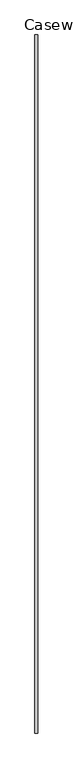
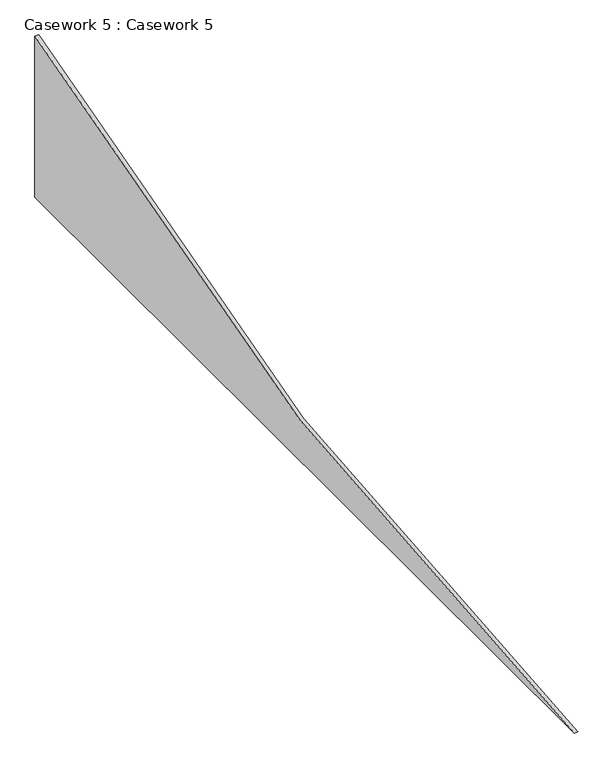
"""IFC4 building model written with IfcOpenShell, lengths in millimetres: furniture geometry, Casework 5 : Casework 5."""

from ifc_helpers import new_model, si_unit, point, frame, frame_2d, origin, place, context, project, spatial, polyline, circle_curve, trimmed, segment, composite_curve, outline, extrude, source, transform, mapped, element, save


def casework_5_casework_5_bcf4e650(model_context):
    return source(origin(), model_context, "Body", "SweptSolid", [
        extrude(outline(composite_curve([segment(polyline([(12368.6757925, 4114.8), (-432.9242075, 4114.8)]), True, "CONTINUOUS"), segment(trimmed(circle_curve(frame_2d((-432.9242075, 40350.6467841)), 36235.8467841), [point((-432.9242075, 4114.8))], [point((12368.6757925, 6451.4487169))], True, "CARTESIAN"), True, "CONTINUOUS"), segment(polyline([(12368.6757925, 6451.4487169), (12368.6757925, 4114.8)]), True, "CONTINUOUS")], self_intersect=False)), frame((2760.8501403, 0.0, 0.0), z_axis=(1.0, 0.0, 0.0), x_axis=(0.0, 1.0, 0.0)), (0.0, 0.0, 1.0), 50.8),
    ])


if __name__ == "__main__":
    model = new_model("IFC4")
    model_context = context("Model", 3, world=origin())
    ifc_project = project(units=[si_unit("LENGTHUNIT", "METRE", prefix="MILLI")], contexts=[model_context])
    site = spatial("IfcSite", under=ifc_project)
    building = spatial("IfcBuilding", under=site)
    placement = place(None, origin())
    casework_5_casework_5_shape = casework_5_casework_5_bcf4e650(model_context)
    element("IfcFurniture", 1, ObjectType="Casework 5 : Casework 5", at=placement, inside=building, context=model_context, shape_type="MappedRepresentation", body=[
        mapped(casework_5_casework_5_shape, transform((0.0, 0.0, 0.0), x_axis=(1.0, 0.0, 0.0), y_axis=(0.0, 1.0, 0.0), z_axis=(0.0, 0.0, 1.0))),
    ])
    save(model, "model.ifc")

# Revit data of these elements
# Element 1 (IfcFurniture, "Casework 5 : Casework 5")
#   Materials on its faces: "Linen, White"
# Materials
#   "Linen, White": class "Textile", colour RGB 247 247 239, transparency 0, Description = "Linen, white", Cost = 0
